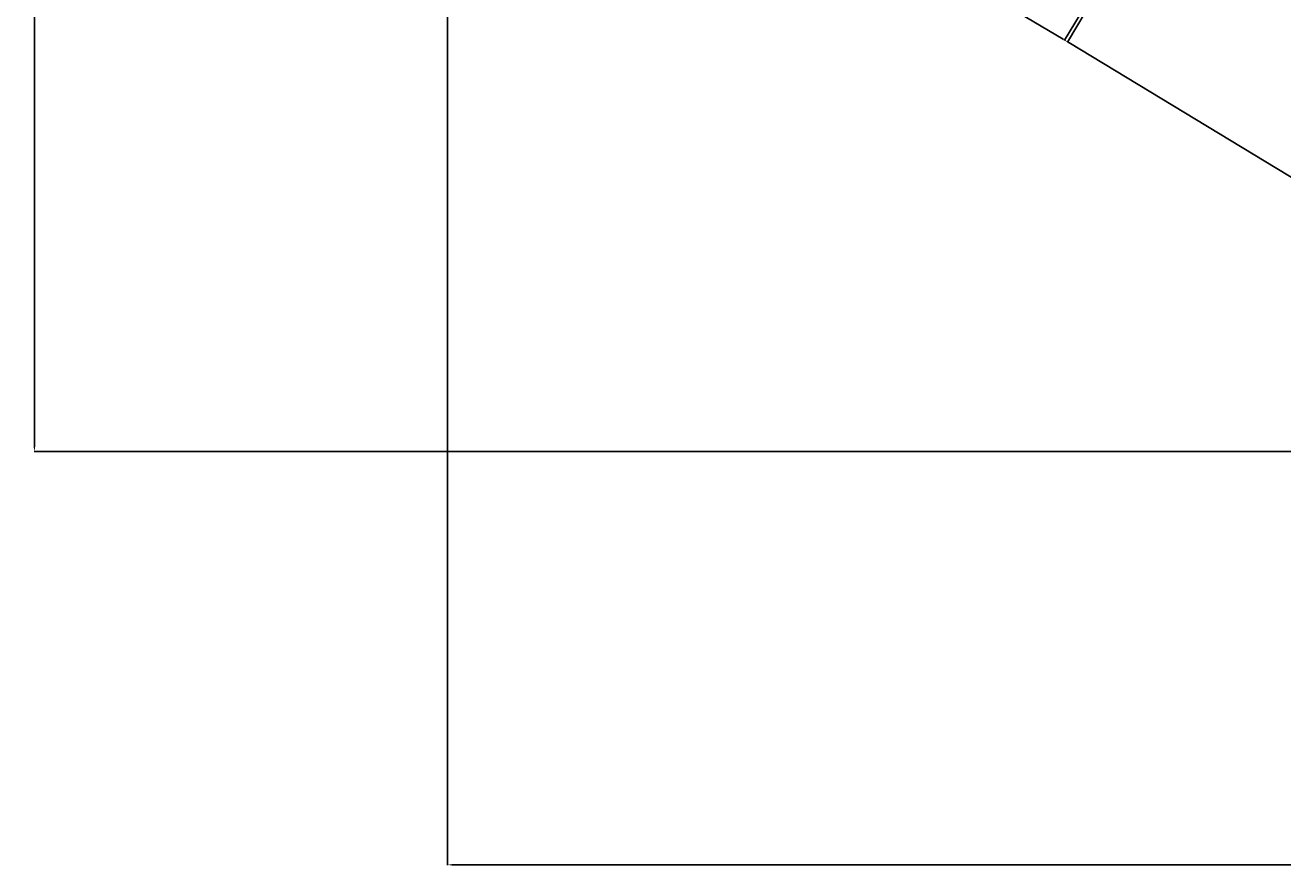
# Model space of a CAD drawing. Units: metres. Extents: x -2391 to 4922, y -635 to 4845.
# Tile 1 of 37: x -2391 to -1367, y -635 to 53. Entities that reach past the tile are written whole.
import ezdxf

# ---------------------------------------------------------------- set-up
doc = ezdxf.new("R2010")
doc.units = ezdxf.units.M
doc.header["$MEASUREMENT"] = 0
doc.layers.add('A-ANNO-DIMS', color=2, linetype='Continuous', lineweight=18)
doc.styles.get("Standard").update_dxf_attribs({"font": 'arial.ttf'})
doc.dimstyles.get("Standard").update_dxf_attribs({"dimtxt": 5, "dimasz": 4, "dimexe": 0.18, "dimexo": 0.0625, "dimgap": 0.09, "dimtad": 0, "dimtih": 1, "dimtoh": 1, "dimdec": 0, "dimzin": 0, "dimdsep": 46, "dimtxsty": 'Standard', "dimcen": 0.09, "dimadec": 0, "dimazin": 0, "dimtfac": 1, "dimtdec": 0, "dimtofl": 0, "dimtmove": 0, "dimatfit": 3, "dimfxl": 1, "dimtolj": 1, "dimtzin": 0, "dimarcsym": 0})

# ---------------------------------------------------------------- blocks, each defined once
blk = doc.blocks.new('*D8')
at = {"layer": 'A-ANNO-DIMS', "color": 0, "lineweight": -2, "transparency": 16777216}
for p, q in [((-2047.3, 3005.2), (-2047.3, -631.4)), ((4577.8, 2350.2), (4577.8, -631.4)), ((-2043.3, -631.2), (1257.6, -631.2)), ((4573.8, -631.2), (1272.8, -631.2))]:
    blk.add_line(p, q, dxfattribs=at)
at = {"layer": 'A-ANNO-DIMS', "color": 0, "transparency": 16777216}
for points in [[(-2043.3, -630.6), (-2043.3, -631.9), (-2047.3, -631.2)], [(4573.8, -630.6), (4573.8, -631.9), (4577.8, -631.2)]]:
    blk.add_solid(points, dxfattribs=at)
at = {"layer": 'Defpoints', "color": 0, "transparency": 16777216}
for p in [(-2047.3, 3005.3), (4577.8, 2350.3), (4577.8, -631.2)]:
    blk.add_point(p, dxfattribs=at)
at = {"layer": 'A-ANNO-DIMS', "color": 0, "transparency": 16777216, "insert": (1265.2, -631.2), "char_height": 5, "attachment_point": 5}
blk.add_mtext('\\A1;6625', dxfattribs=at)
blk = doc.blocks.new('*D10')
at = {"layer": 'A-ANNO-DIMS', "color": 0, "lineweight": -2, "transparency": 16777216}
for p, q in [((550.7, 4505.3), (-2384, 4505.3)), ((-2383.8, 4501.3), (-2383.8, 2107.9)), ((-2383.8, -290.7), (-2383.8, 2102.6)), ((-488.6, -294.7), (-2384, -294.7))]:
    blk.add_line(p, q, dxfattribs=at)
at = {"layer": 'A-ANNO-DIMS', "color": 0, "transparency": 16777216}
for points in [[(-2384.5, 4501.3), (-2383.2, 4501.3), (-2383.8, 4505.3)], [(-2384.5, -290.7), (-2383.2, -290.7), (-2383.8, -294.7)]]:
    blk.add_solid(points, dxfattribs=at)
at = {"layer": 'Defpoints', "color": 0, "transparency": 16777216}
for p in [(-2383.8, 4505.3), (550.7, 4505.3), (-488.5, -294.7)]:
    blk.add_point(p, dxfattribs=at)
at = {"layer": 'A-ANNO-DIMS', "color": 0, "transparency": 16777216, "insert": (-2383.8, 2105.3), "char_height": 5, "attachment_point": 5}
blk.add_mtext('\\A1;4800', dxfattribs=at)
blk = doc.blocks.new('*D50')
at = {"layer": 'A-ANNO-DIMS', "color": 0, "lineweight": -2, "transparency": 16777216}
for p, q in [((-1757.3, 558), (-1929.2, 268.6)), ((-1370.5, 328.3), (-1542.4, 38.9)), ((-1925.6, 266.7), (-1740.1, 156.5)), ((-1545.8, 41.1), (-1731.3, 151.2))]:
    blk.add_line(p, q, dxfattribs=at)
at = {"layer": 'A-ANNO-DIMS', "color": 0, "transparency": 16777216}
for points in [[(-1925.3, 267.3), (-1926, 266.1), (-1929.1, 268.7)], [(-1545.4, 41.6), (-1546.1, 40.5), (-1542.3, 39)]]:
    blk.add_solid(points, dxfattribs=at)
at = {"layer": 'Defpoints', "color": 0, "transparency": 16777216}
for p in [(-1757.2, 558.1), (-1370.5, 328.3), (-1929.1, 268.7)]:
    blk.add_point(p, dxfattribs=at)
at = {"layer": 'A-ANNO-DIMS', "color": 0, "transparency": 16777216, "insert": (-1735.7, 153.9), "char_height": 5, "attachment_point": 5}
blk.add_mtext('\\A1;449.8', dxfattribs=at)
blk = doc.blocks.new('*D51')
at = {"layer": 'A-ANNO-DIMS', "color": 0, "lineweight": -2, "transparency": 16777216}
for p, q in [((-1370.5, 328.3), (-1544.9, 40.4)), ((-1541.4, 38.4), (-1301.9, -106.6)), ((-876, 28.7), (-1050.4, -259.2)), ((-1053.8, -257), (-1293.2, -111.9))]:
    blk.add_line(p, q, dxfattribs=at)
at = {"layer": 'A-ANNO-DIMS', "color": 0, "transparency": 16777216}
for points in [[(-1541.1, 39), (-1541.8, 37.9), (-1544.8, 40.5)], [(-1053.4, -256.4), (-1054.1, -257.5), (-1050.3, -259)]]:
    blk.add_solid(points, dxfattribs=at)
at = {"layer": 'Defpoints', "color": 0, "transparency": 16777216}
for p in [(-1370.5, 328.3), (-1544.8, 40.5), (-876, 28.8)]:
    blk.add_point(p, dxfattribs=at)
at = {"layer": 'A-ANNO-DIMS', "color": 0, "transparency": 16777216, "insert": (-1297.6, -109.3), "char_height": 5, "attachment_point": 5}
blk.add_mtext('\\A1;578.1', dxfattribs=at)

msp = doc.modelspace()

# ---------------------------------------------------------------- dimensions: what is measured, and where the dimension line sits
at = {"layer": 'A-ANNO-DIMS'}
for base, p1, p2, angle, override, picture, middle in [((-2383.8343, 4505.2763), (-488.4886, -294.7237), (550.7419, 4505.2763), 90, {"dimdec": 0, "dimlfac": 1, "dimrnd": 0, "dimzin": 0, "dimdsep": 46, "dimlunit": 2}, '*D10', (-2383.8343, 2105.2763)), ((-1929.0761, 268.7454), (-1370.4753, 328.3288), (-1757.2287, 558.0561), 149.2901447, {"dimdec": 1, "dimlfac": 1, "dimrnd": 0, "dimzin": 0, "dimdsep": 46, "dimlunit": 2}, '*D50', (-1735.6994, 153.8817)), ((-1544.828, 40.5209), (-875.9874, 28.7702), (-1370.4753, 328.3288), 148.7927031, {"dimdec": 1, "dimlfac": 1, "dimrnd": 0, "dimzin": 0, "dimdsep": 46, "dimlunit": 2}, '*D51', (-1297.5841, -109.2584))]:
    dim = msp.add_linear_dim(base=base, p1=p1, p2=p2, angle=angle, dimstyle='Standard', override=override, dxfattribs=at)
    dim.commit()
    dim.dimension.update_dxf_attribs({"geometry": picture, "text_midpoint": middle})
dim = msp.add_linear_dim(base=(4577.76, -631.2237), p1=(-2047.3343, 3005.2763), p2=(4577.76, 2350.2763), dimstyle='Standard', override={"dimdec": 0, "dimlfac": 1, "dimrnd": 0, "dimzin": 0, "dimdsep": 46, "dimlunit": 2}, dxfattribs=at)
dim.commit()
dim.dimension.update_dxf_attribs({"geometry": '*D8', "text_midpoint": (1265.2128, -631.2237)})

doc.saveas('drawing.dxf')
